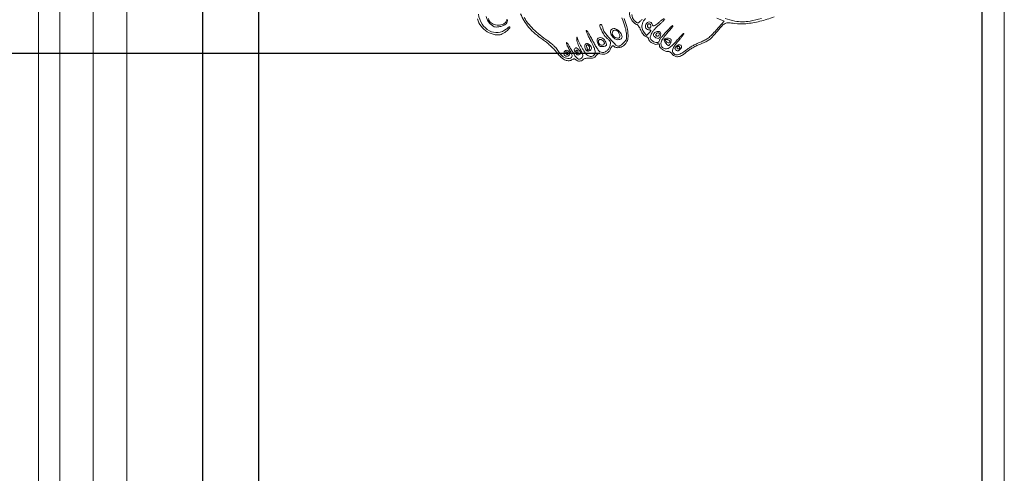
# Model space of a CAD drawing. Units: inches. Extents: x 2656 to 9931, y 1941 to 3068.
# Tile 31 of 46: x 2817 to 2868, y 2929 to 2952. Entities that reach past the tile are written whole.
import ezdxf

# ---------------------------------------------------------------- set-up
doc = ezdxf.new("R2010")
doc.units = ezdxf.units.IN
for name, color, linetype, lineweight in [('A-ANNO-DIMS', 2, 'Continuous', 18), ('A-ELEV-FNSH', 8, 'Continuous', 13), ('A-ELEV-ORN', 8, 'Continuous', 13)]:
    doc.layers.add(name, color=color, linetype=linetype, lineweight=lineweight)
doc.styles.get("Standard").update_dxf_attribs({"font": 'arial.ttf'})
doc.dimstyles.new('ISO-25', dxfattribs={"dimtxt": 6, "dimasz": 2.5, "dimexe": 1.25, "dimexo": 0.625, "dimtad": 1, "dimdec": 0, "dimlunit": 3, "dimtxsty": 'Standard', "dimcen": 2.5, "dimadec": 0, "dimazin": 0, "dimtfac": 1, "dimtdec": 0, "dimtmove": 0, "dimatfit": 3, "dimfxl": 1, "dimarcsym": 0})

# ---------------------------------------------------------------- blocks, each defined once
blk = doc.blocks.new('*D151')
at = {"layer": 'A-ANNO-DIMS', "color": 0, "lineweight": -2, "transparency": 16777216}
for p, q in [((2829.546, 2956.424), (2829.546, 2703.709)), ((2867.059, 2955.98), (2867.059, 2703.709)), ((2832.046, 2704.959), (2864.559, 2704.959))]:
    blk.add_line(p, q, dxfattribs=at)
at = {"layer": 'A-ANNO-DIMS', "color": 0, "transparency": 16777216}
for points in [[(2832.046, 2705.376), (2832.046, 2704.543), (2829.546, 2704.959)], [(2864.559, 2705.376), (2864.559, 2704.543), (2867.059, 2704.959)]]:
    blk.add_solid(points, dxfattribs=at)
at = {"layer": 'Defpoints', "color": 0, "transparency": 16777216}
for p in [(2829.546, 2957.049), (2867.059, 2956.605), (2867.059, 2704.959)]:
    blk.add_point(p, dxfattribs=at)
at = {"layer": 'A-ANNO-DIMS', "color": 0, "transparency": 16777216, "insert": (2848.302, 2708.689), "char_height": 6, "attachment_point": 5}
blk.add_mtext('3\'-1 1/2"', dxfattribs=at)
blk = doc.blocks.new('*D152')
at = {"layer": 'A-ANNO-DIMS', "color": 0, "lineweight": -2, "transparency": 16777216}
for p, q in [((2847.28, 2990.828), (2707.323, 2990.828)), ((2708.573, 2988.328), (2708.573, 2952.971)), ((2847.248, 2950.471), (2707.323, 2950.471))]:
    blk.add_line(p, q, dxfattribs=at)
at = {"layer": 'A-ANNO-DIMS', "color": 0, "transparency": 16777216}
for points in [[(2708.156, 2988.328), (2708.989, 2988.328), (2708.573, 2990.828)], [(2708.156, 2952.971), (2708.989, 2952.971), (2708.573, 2950.471)]]:
    blk.add_solid(points, dxfattribs=at)
at = {"layer": 'Defpoints', "color": 0, "transparency": 16777216}
for p in [(2847.905, 2990.828), (2708.573, 2950.471), (2847.873, 2950.471)]:
    blk.add_point(p, dxfattribs=at)
at = {"layer": 'A-ANNO-DIMS', "color": 0, "transparency": 16777216, "insert": (2704.843, 2970.649), "char_height": 6, "attachment_point": 5, "rotation": 90}
blk.add_mtext('3\'-4 1/2"', dxfattribs=at)
blk = doc.blocks.new('*D153')
at = {"layer": 'A-ANNO-DIMS', "color": 0, "lineweight": -2, "transparency": 16777216}
for p, q in [((2826.64, 2993.722), (2826.64, 2703.709)), ((2829.546, 2956.424), (2829.546, 2703.709)), ((2824.14, 2704.959), (2821.64, 2704.959)), ((2826.64, 2704.959), (2829.546, 2704.959)), ((2832.046, 2704.959), (2851.745, 2704.959))]:
    blk.add_line(p, q, dxfattribs=at)
at = {"layer": 'A-ANNO-DIMS', "color": 0, "transparency": 16777216}
for points in [[(2824.14, 2705.376), (2824.14, 2704.543), (2826.64, 2704.959)], [(2832.046, 2705.376), (2832.046, 2704.543), (2829.546, 2704.959)]]:
    blk.add_solid(points, dxfattribs=at)
at = {"layer": 'Defpoints', "color": 0, "transparency": 16777216}
for p in [(2826.64, 2994.347), (2829.546, 2957.049), (2829.546, 2704.959)]:
    blk.add_point(p, dxfattribs=at)
at = {"layer": 'A-ANNO-DIMS', "color": 0, "transparency": 16777216, "insert": (2843.145, 2708.65), "char_height": 6, "attachment_point": 5}
blk.add_mtext('0\'-3"', dxfattribs=at)

msp = doc.modelspace()

# ---------------------------------------------------------------- linework, layer by layer
at = {"layer": 'A-ELEV-FNSH'}
for p, q in [((2818.129, 2887.893), (2818.129, 2998.286)), ((2819.227, 2887.893), (2819.227, 2998.286)), ((2820.954, 2887.893), (2820.954, 2998.286)), ((2822.705, 2887.893), (2822.705, 2998.286))]:
    msp.add_line(p, q, dxfattribs=at)
msp.add_lwpolyline([(2826.64, 2994.347), (2868.226, 2994.347), (2868.226, 2892.035), (2826.64, 2892.035)], close=True, dxfattribs=at)
at = {"layer": 'A-ELEV-ORN'}
for points in [[(2848.801, 2952.672, 0.216659), (2848.924, 2952.173, 0.024142), (2848.989, 2952.098, 0.029169), (2849.056, 2952.036, 0.030018), (2849.118, 2951.991, 0.14114), (2849.16, 2951.978, -0.206861), (2849.199, 2951.961, -0.032643), (2849.253, 2951.894, -0.031638), (2849.311, 2951.801, -0.022863), (2849.363, 2951.691, 0.032088), (2849.421, 2951.575, 0.039321), (2849.49, 2951.475, 0.044219), (2849.561, 2951.401, 0.114242), (2849.627, 2951.367, -0.05877), (2849.681, 2951.346, -0.064566), (2849.728, 2951.313, -0.073322), (2849.759, 2951.273, -0.133163), (2849.77, 2951.234, 0.196142), (2849.812, 2951.132, 0.063805), (2849.942, 2951.029, 0.063115), (2850.097, 2950.961, 0.16535), (2850.217, 2950.965, -0.060457), (2850.268, 2950.978, -0.16436), (2850.304, 2950.971, -0.184298), (2850.325, 2950.944, -0.078925), (2850.333, 2950.898, 0.185704), (2850.373, 2950.794, 0.054155), (2850.503, 2950.678, 0.054153), (2850.655, 2950.593, 0.183335), (2850.767, 2950.588, -0.170308), (2850.81, 2950.587, -0.049123), (2850.872, 2950.558, -0.043275), (2850.94, 2950.508, -0.034537), (2851.003, 2950.443, 0.112897), (2851.154, 2950.332, 0.151039), (2851.321, 2950.314, 0.097306), (2851.525, 2950.396, 0.029789), (2851.794, 2950.595, -0.032237), (2851.932, 2950.696, -0.016051), (2852.119, 2950.806, -0.015862), (2852.32, 2950.909, -0.022458), (2852.506, 2950.986, 0.023761), (2852.744, 2951.086, 0.048062), (2852.919, 2951.191, 0.044595), (2853.078, 2951.332, 0.017836), (2853.27, 2951.551, -0.01156), (2853.571, 2951.903, -0.094216), (2853.738, 2952.03, -0.127885), (2853.919, 2952.069, -0.028057), (2854.239, 2952.037, 0.065509), (2854.825, 2952.022, 0.033923), (2855.548, 2952.148, 0.033055), (2856.284, 2952.381, 0.043026)], [(2840.893, 2952.277, 0.097952), (2841.082, 2951.892, 0.097989), (2841.403, 2951.609, 0.086415), (2841.822, 2951.453, 0.039063), (2841.956, 2951.439, 0.065886), (2842.068, 2951.451, 0.061015), (2842.178, 2951.492, 0.028884), (2842.309, 2951.57, 0.020818), (2842.404, 2951.64, 0.022925), (2842.489, 2951.715, 0.023115), (2842.555, 2951.786, 0.097823), (2842.584, 2951.836, 0.416465), (2842.574, 2951.856, 0.186344), (2842.542, 2951.854, 0.050913), (2842.477, 2951.816, 0.01734), (2842.39, 2951.748, -0.149603), (2841.966, 2951.568, -0.150262), (2841.514, 2951.656, -0.129848), (2841.142, 2952.002, -0.100707), (2840.945, 2952.522, -0.033876)], [(2841.353, 2952.403, 0.154333), (2841.544, 2952.035, 0.024688), (2841.669, 2951.922, 0.082141), (2841.765, 2951.867, 0.092986), (2841.866, 2951.849, 0.037226), (2842.007, 2951.862, 0.038366), (2842.202, 2951.909, 0.07779), (2842.341, 2951.979, 0.107669), (2842.424, 2952.071, 0.139876), (2842.451, 2952.181, 0.032838), (2842.446, 2952.228, 0.51286), (2842.433, 2952.234, 0.163716), (2842.416, 2952.216, 0.010729), (2842.386, 2952.146, -0.203512), (2842.242, 2952.003, -0.096781), (2841.981, 2951.952, -0.091076), (2841.705, 2952.003, -0.155421), (2841.524, 2952.148, -0.129288), (2841.477, 2952.285, -0.032632)], [(2843.136, 2952.533, 0.048744), (2843.312, 2952.178, 0.037984), (2843.567, 2951.831, 0.035321), (2843.893, 2951.502, 0.029786), (2844.28, 2951.201, -0.019345), (2844.472, 2951.059, -0.014584), (2844.672, 2950.888, -0.014803), (2844.851, 2950.716, -0.032702), (2844.974, 2950.572, 0.035674), (2845.196, 2950.317, 0.072427), (2845.41, 2950.158, 0.10378), (2845.604, 2950.101, 0.161146), (2845.773, 2950.142, -0.035481), (2845.845, 2950.18, -0.087902), (2845.902, 2950.194, -0.117123), (2845.951, 2950.186, -0.096474), (2845.994, 2950.156, 0.107887), (2846.08, 2950.101, 0.095562), (2846.186, 2950.083, 0.093343), (2846.292, 2950.106, 0.097186), (2846.381, 2950.166, -0.108118), (2846.431, 2950.198, -0.038631), (2846.512, 2950.221, -0.036146), (2846.608, 2950.233, -0.035408), (2846.705, 2950.232, 0.035182), (2846.823, 2950.23, 0.075501), (2846.912, 2950.248, 0.087997), (2846.983, 2950.29, 0.063219), (2847.045, 2950.358, -0.05042), (2847.096, 2950.417, -0.079909), (2847.151, 2950.455, -0.095326), (2847.208, 2950.47, -0.106795), (2847.263, 2950.461, 0.103678), (2847.42, 2950.436, 0.099264), (2847.576, 2950.475, 0.095648), (2847.71, 2950.573, 0.088752), (2847.802, 2950.716, -0.023551), (2847.847, 2950.812, -0.092945), (2847.888, 2950.863, -0.202519), (2847.926, 2950.876, -0.176634), (2847.965, 2950.858, 0.148207), (2848.095, 2950.789, 0.097714), (2848.265, 2950.788, 0.087841), (2848.438, 2950.855, 0.090106), (2848.576, 2950.977, 0.044786), (2848.653, 2951.094, 0.069827), (2848.694, 2951.207, 0.054055), (2848.708, 2951.347, 0.017152), (2848.7, 2951.557, 0.049543), (2848.643, 2951.884, 0.023015), (2848.508, 2952.294, 0.022134)], [(2848.393, 2952.319, -0.01692), (2848.543, 2951.895, -0.043427), (2848.613, 2951.578, -0.015509), (2848.635, 2951.365, -0.077549), (2848.625, 2951.245, -0.100968), (2848.58, 2951.149, -0.035807), (2848.48, 2951.035, -0.019689), (2848.405, 2950.965, -0.02395), (2848.33, 2950.907, -0.023531), (2848.263, 2950.865, -0.129915), (2848.222, 2950.854, -0.20167), (2848.082, 2950.912, -0.012833), (2847.774, 2951.244, -0.016262), (2847.489, 2951.588, -0.115769), (2847.4, 2951.784, 0.028588), (2847.381, 2951.859, 0.041166), (2847.354, 2951.922, 0.047726), (2847.326, 2951.966, 0.229861), (2847.299, 2951.979, 0.186476), (2847.258, 2951.963, 0.246151), (2847.244, 2951.926, 0.060512), (2847.265, 2951.845, 0.005494), (2847.343, 2951.653, 0.03364), (2847.396, 2951.547, 0.023761), (2847.469, 2951.435, 0.02409), (2847.549, 2951.335, 0.045688), (2847.624, 2951.264, -0.049294), (2847.74, 2951.152, -0.129909), (2847.79, 2951.049, -0.118001), (2847.785, 2950.928, -0.037071), (2847.722, 2950.758, -0.093173), (2847.636, 2950.636, -0.099676), (2847.513, 2950.557, -0.104799), (2847.375, 2950.534, -0.113979), (2847.244, 2950.57, -0.113308), (2847.186, 2950.621, -0.011986), (2847.085, 2950.77, -0.014319), (2846.972, 2950.956, -0.011031), (2846.859, 2951.166, 0.007389), (2846.751, 2951.369, 0.012759), (2846.655, 2951.534, 0.006744), (2846.572, 2951.664, 0.475628), (2846.55, 2951.666, 0.298473), (2846.543, 2951.636, 0.005773), (2846.605, 2951.485, 0.011889), (2846.685, 2951.306, 0.007437), (2846.787, 2951.101, -0.008452), (2846.924, 2950.823, -0.037472), (2846.99, 2950.653, -0.069448), (2847.008, 2950.536, -0.145257), (2846.983, 2950.448, -0.146465), (2846.856, 2950.337, -0.198924), (2846.705, 2950.332, -0.123587), (2846.539, 2950.447, -0.046452), (2846.372, 2950.678, -0.009207), (2846.288, 2950.825, -0.008845), (2846.209, 2950.978, -0.008807), (2846.143, 2951.115, -0.0314), (2846.109, 2951.205, 0.002514), (2846.074, 2951.317, 0.226761), (2846.062, 2951.33, 0.508235), (2846.053, 2951.324, 0.004483), (2846.048, 2951.229, 0.07523), (2846.057, 2951.147, 0.017337), (2846.098, 2951.014, 0.017529), (2846.156, 2950.862, 0.016323), (2846.226, 2950.711, -0.008903), (2846.33, 2950.495, -0.068964), (2846.362, 2950.387, -0.146939), (2846.351, 2950.312, -0.089299), (2846.299, 2950.237, -0.17255), (2846.191, 2950.185, -0.201973), (2846.083, 2950.218, -0.077507), (2845.955, 2950.364, -0.013086), (2845.764, 2950.684, 0.008257), (2845.622, 2950.925, 0.047089), (2845.533, 2951.044, 0.715316), (2845.51, 2951.034, 0.071182), (2845.53, 2950.942, 0.021409), (2845.557, 2950.879, 0.006729), (2845.602, 2950.788, 0.006709), (2845.655, 2950.688, 0.007384), (2845.71, 2950.592, -0.041313), (2845.792, 2950.421, -0.176517), (2845.794, 2950.309, -0.238643), (2845.726, 2950.243, -0.075156), (2845.581, 2950.221, -0.103457), (2845.441, 2950.25, -0.071525), (2845.303, 2950.335, -0.055375), (2845.166, 2950.479, -0.028769), (2845.026, 2950.686, 0.053224), (2844.955, 2950.781, 0.018463), (2844.834, 2950.902, 0.0181), (2844.69, 2951.026, 0.020079), (2844.542, 2951.135, -0.021598), (2844.142, 2951.432, -0.025464), (2843.792, 2951.747, -0.027925), (2843.511, 2952.059, -0.051755), (2843.327, 2952.345, -0.041492)], [(2849.443, 2952.253, -0.031818), (2849.345, 2952.153, -0.02297), (2849.253, 2952.076, -0.18391), (2849.201, 2952.061, -0.160327), (2849.148, 2952.084, -0.016424), (2849.048, 2952.178, -0.185893), (2848.905, 2952.5, -0.094612)], [(2850.574, 2952.297, 0.028686), (2850.476, 2952.229, 0.011691), (2850.351, 2952.127, -0.006102), (2850.146, 2951.956, -0.080138), (2850.061, 2951.907, -0.286715), (2850.008, 2951.918, -0.11616), (2849.966, 2951.981, 0.117291), (2849.902, 2952.078, 0.182702), (2849.811, 2952.115, 0.173341), (2849.714, 2952.083, 0.105255), (2849.635, 2951.99, 0.123366), (2849.609, 2951.886, 0.148353), (2849.638, 2951.789, 0.140375), (2849.718, 2951.722, 0.106459), (2849.83, 2951.698, -0.097174), (2849.872, 2951.69, -0.360986), (2849.884, 2951.667, -0.11978), (2849.865, 2951.627, -0.014081), (2849.8, 2951.552), (2849.668, 2951.405), (2849.543, 2951.559, -0.11694), (2849.432, 2951.789, -0.142406), (2849.449, 2952.027, -0.093777), (2849.607, 2952.292, -0.031312)], [(2853.322, 2952.304), (2853.698, 2952.151), (2853.279, 2951.683, -0.014019), (2853.048, 2951.439, -0.035056), (2852.863, 2951.278, -0.042181), (2852.679, 2951.163, -0.030354), (2852.458, 2951.065, 0.020169), (2852.285, 2950.992, 0.014439), (2852.097, 2950.899, 0.014617), (2851.924, 2950.799, 0.030123), (2851.796, 2950.708, -0.023096), (2851.542, 2950.525, -0.065579), (2851.346, 2950.43, -0.108644), (2851.194, 2950.415, -0.169259), (2851.076, 2950.472, -0.14578), (2851.018, 2950.581, -0.143269), (2851.027, 2950.705, -0.069423), (2851.119, 2950.873, -0.01412), (2851.33, 2951.14, 0.007738), (2851.433, 2951.267, 0.011134), (2851.52, 2951.382, 0.007109), (2851.588, 2951.481, 0.149256), (2851.599, 2951.515, 0.659704), (2851.585, 2951.521, 0.007404), (2851.49, 2951.427, 0.010983), (2851.371, 2951.301, 0.005888), (2851.229, 2951.141, -0.022729), (2850.977, 2950.874, -0.083791), (2850.786, 2950.743, -0.155343), (2850.629, 2950.723, -0.15181), (2850.487, 2950.797, -0.144109), (2850.418, 2950.924, -0.132791), (2850.426, 2951.073, -0.077589), (2850.521, 2951.26, -0.023454), (2850.719, 2951.509, 0.002598), (2851.017, 2951.853, 0.277519), (2851.026, 2951.911, 0.545774), (2850.99, 2951.918, 0.002794), (2850.684, 2951.599, 0.009193), (2850.55, 2951.451, 0.013114), (2850.436, 2951.315, 0.009044), (2850.347, 2951.198, 0.159361), (2850.333, 2951.153, -0.217862), (2850.298, 2951.077, -0.162357), (2850.211, 2951.041, -0.109971), (2850.09, 2951.06, -0.078028), (2849.972, 2951.128, -0.033256), (2849.885, 2951.209, -0.145423), (2849.854, 2951.271, -0.122821), (2849.858, 2951.345, -0.020849), (2849.908, 2951.48, -0.053925), (2849.964, 2951.583, -0.021987), (2850.062, 2951.711, -0.021448), (2850.179, 2951.84, -0.02561), (2850.301, 2951.951, 0.013398), (2850.419, 2952.053, 0.015652), (2850.525, 2952.156, 0.014705), (2850.609, 2952.248, 0.085937)], [(2855.626, 2952.288, -0.01477), (2855.041, 2952.158, -0.047431), (2854.644, 2952.12, -0.052476), (2854.249, 2952.161, -0.023008), (2853.739, 2952.294, -0.023068)]]:
    msp.add_lwpolyline(points, format="xyb", dxfattribs=at)
for points in [[(2847.847, 2951.721, 0.251131), (2847.798, 2951.559, 0.124898), (2847.894, 2951.359, 0.113091), (2848.082, 2951.216, 0.200091), (2848.274, 2951.21, 0.048277), (2848.344, 2951.245, 0.117693), (2848.384, 2951.286, 0.140447), (2848.397, 2951.335, 0.081949), (2848.387, 2951.396, 0.077801), (2848.283, 2951.587, 0.09434), (2848.132, 2951.723, 0.124914), (2847.974, 2951.77, 0.210773)], [(2848.22, 2951.562, -0.03358), (2848.28, 2951.43, -0.141285), (2848.286, 2951.344, -0.241436), (2848.246, 2951.294, -0.105107), (2848.161, 2951.276, -0.117324), (2848.044, 2951.304, -0.10171), (2847.945, 2951.382, -0.109775), (2847.89, 2951.487, -0.158111), (2847.896, 2951.591, -0.149626), (2847.957, 2951.669, -0.177198), (2848.047, 2951.693, -0.148121), (2848.144, 2951.654, -0.100327)], [(2849.875, 2951.838, -0.074012), (2849.849, 2951.807, -0.156529), (2849.82, 2951.794, -0.15302), (2849.788, 2951.801, -0.06978), (2849.754, 2951.826, -0.088981), (2849.731, 2951.859, -0.076381), (2849.719, 2951.9, -0.077007), (2849.721, 2951.942, -0.093176), (2849.735, 2951.979, -0.074012), (2849.761, 2952.011, -0.156529), (2849.791, 2952.023, -0.15302), (2849.822, 2952.017, -0.06978), (2849.856, 2951.991, -0.088981), (2849.879, 2951.958, -0.076381), (2849.891, 2951.917, -0.077007), (2849.89, 2951.875, -0.093176)], [(2847.166, 2951.275, 0.095208), (2847.122, 2951.235, 0.133582), (2847.103, 2951.185, 0.088345), (2847.108, 2951.117, 0.025322), (2847.139, 2951.016, 0.039226), (2847.182, 2950.92, 0.106844), (2847.231, 2950.865, 0.12504), (2847.293, 2950.839, 0.064245), (2847.378, 2950.838, 0.021524), (2847.516, 2950.859, 0.175493), (2847.569, 2950.892, 0.215239), (2847.583, 2950.947, 0.033952), (2847.556, 2951.06, 0.092865), (2847.491, 2951.18, 0.097317), (2847.388, 2951.267, 0.110796), (2847.271, 2951.301, 0.15554)], [(2847.441, 2951.109, -0.052573), (2847.475, 2951.059, -0.14188), (2847.483, 2951.017, -0.144742), (2847.468, 2950.978, -0.055548), (2847.427, 2950.935, -0.17181), (2847.345, 2950.905, -0.155184), (2847.258, 2950.931, -0.13098), (2847.191, 2951.009, -0.112001), (2847.168, 2951.114, -0.218344), (2847.197, 2951.177, -0.184093), (2847.266, 2951.202, -0.123773), (2847.359, 2951.177, -0.092306)], [(2850.06, 2951.533, 0.078467), (2850.029, 2951.481, 0.152913), (2850.026, 2951.433, 0.116494), (2850.05, 2951.384, 0.035989), (2850.109, 2951.323, 0.119877), (2850.213, 2951.266, 0.20352), (2850.31, 2951.28, 0.172143), (2850.379, 2951.364, 0.086245), (2850.403, 2951.501, 0.208669), (2850.366, 2951.585, 0.165357), (2850.275, 2951.626, 0.127666), (2850.158, 2951.606, 0.116165)], [(2850.333, 2951.498, -0.108877), (2850.319, 2951.438, -0.127543), (2850.282, 2951.393, -0.144342), (2850.232, 2951.375, -0.153624), (2850.181, 2951.388, -0.216101), (2850.152, 2951.431, -0.159804), (2850.161, 2951.489, -0.132181), (2850.205, 2951.539, -0.145303), (2850.266, 2951.557, -0.087308), (2850.292, 2951.553, -0.094392), (2850.313, 2951.54, -0.100145), (2850.328, 2951.521, -0.112153)], [(2850.58, 2951.208, 0.193695), (2850.574, 2951.172, 0.058266), (2850.592, 2951.119, 0.048819), (2850.629, 2951.058, 0.036452), (2850.68, 2950.999, 0.010243), (2850.775, 2950.907, 0.186958), (2850.813, 2950.892, 0.256873), (2850.845, 2950.91, 0.019698), (2850.897, 2950.997, 0.040391), (2850.923, 2951.056, 0.043863), (2850.938, 2951.117, 0.048392), (2850.941, 2951.171, 0.129399), (2850.93, 2951.207, 0.180632), (2850.865, 2951.257, 0.074944), (2850.755, 2951.274, 0.075027), (2850.645, 2951.257, 0.182191)], [(2850.857, 2951.14, -0.189332), (2850.869, 2951.076, -0.296611), (2850.831, 2951.037, -0.169397), (2850.755, 2951.045, -0.107759), (2850.684, 2951.101, -0.020503), (2850.641, 2951.157, -0.209835), (2850.635, 2951.185, -0.309419), (2850.652, 2951.201, -0.038489), (2850.707, 2951.205, -0.053722), (2850.752, 2951.201, -0.048999), (2850.796, 2951.186, -0.052232), (2850.834, 2951.165, -0.09982)], [(2845.386, 2950.542, 0.166245), (2845.382, 2950.451, 0.151719), (2845.435, 2950.372, 0.149289), (2845.524, 2950.337, 0.16055), (2845.615, 2950.358, 0.190949), (2845.668, 2950.429, 0.143859), (2845.666, 2950.528, 0.139493), (2845.61, 2950.611, 0.178716), (2845.524, 2950.643, 0.090292), (2845.483, 2950.635, 0.066647), (2845.442, 2950.613, 0.065393), (2845.408, 2950.581, 0.079367)], [(2845.938, 2950.715, 0.198865), (2845.922, 2950.619, 0.09268), (2845.974, 2950.502, 0.097846), (2846.062, 2950.416, 0.240946), (2846.149, 2950.407, 0.087263), (2846.223, 2950.451, 0.223388), (2846.248, 2950.507, 0.153424), (2846.224, 2950.578, 0.038406), (2846.143, 2950.673, 0.013143), (2846.056, 2950.755, 0.133914), (2846.013, 2950.777, 0.254303), (2845.978, 2950.766, 0.055423)], [(2846.113, 2950.572, -0.042167), (2846.11, 2950.545, -0.061769), (2846.103, 2950.523, -0.081139), (2846.093, 2950.507, -0.210953), (2846.082, 2950.502, -0.151918), (2846.067, 2950.507, -0.038439), (2846.047, 2950.523, -0.035638), (2846.026, 2950.545, -0.029505), (2846.007, 2950.572, -0.082592), (2845.996, 2950.599, -0.161196), (2845.998, 2950.622, -0.182303), (2846.013, 2950.637, -0.108972), (2846.038, 2950.643, -0.093332), (2846.066, 2950.637, -0.09642), (2846.091, 2950.622, -0.099167), (2846.107, 2950.599, -0.105053)], [(2846.465, 2950.871, 0.065921), (2846.483, 2950.744, 0.11591), (2846.534, 2950.651, 0.153891), (2846.61, 2950.607, 0.149294), (2846.698, 2950.613, 0.107755), (2846.777, 2950.664, 0.167613), (2846.811, 2950.737, 0.147269), (2846.796, 2950.822, 0.077976), (2846.731, 2950.91, 0.080544), (2846.64, 2950.976, 0.15324), (2846.551, 2950.99, 0.211421), (2846.489, 2950.951, 0.151601)], [(2846.7, 2950.821, -0.066719), (2846.71, 2950.778, -0.072258), (2846.708, 2950.736, -0.081026), (2846.695, 2950.7, -0.126981), (2846.672, 2950.676, -0.034732), (2846.646, 2950.662, -0.074198), (2846.625, 2950.657, -0.143207), (2846.611, 2950.659, -0.287633), (2846.605, 2950.668, 0.061959), (2846.602, 2950.687, 0.00979), (2846.592, 2950.724, 0.010735), (2846.579, 2950.768, 0.009199), (2846.562, 2950.813, -0.054634), (2846.551, 2950.855, -0.098218), (2846.553, 2950.891, -0.14605), (2846.567, 2950.915, -0.188995), (2846.59, 2950.924, -0.125056), (2846.62, 2950.917, -0.064167), (2846.651, 2950.894, -0.057615), (2846.679, 2950.86, -0.055112)], [(2851.184, 2950.828, 0.053545), (2851.151, 2950.777, 0.143201), (2851.143, 2950.735, 0.143819), (2851.158, 2950.696, 0.054184), (2851.2, 2950.652, 0.077176), (2851.253, 2950.621, 0.154286), (2851.3, 2950.617, 0.117177), (2851.35, 2950.642, 0.035256), (2851.412, 2950.701, 0.060425), (2851.475, 2950.791, 0.19481), (2851.483, 2950.862, 0.240731), (2851.44, 2950.908, 0.087827), (2851.349, 2950.924, 0.088999), (2851.311, 2950.917, 0.043202), (2851.266, 2950.896, 0.041019), (2851.221, 2950.865, 0.046615)], [(2851.388, 2950.783, -0.099038), (2851.382, 2950.757, -0.097945), (2851.367, 2950.734, -0.097945), (2851.344, 2950.718, -0.099038), (2851.317, 2950.713, -0.099038), (2851.29, 2950.718, -0.097945), (2851.268, 2950.734, -0.097945), (2851.252, 2950.757, -0.099038), (2851.247, 2950.783, -0.099038), (2851.252, 2950.81, -0.097945), (2851.268, 2950.833, -0.097945), (2851.29, 2950.848, -0.099038), (2851.317, 2950.854, -0.099038), (2851.344, 2950.848, -0.097945), (2851.367, 2950.833, -0.097945), (2851.382, 2950.81, -0.099038)], [(2845.585, 2950.502, -0.082592), (2845.596, 2950.475, -0.161196), (2845.594, 2950.452, -0.182303), (2845.579, 2950.437, -0.108972), (2845.554, 2950.432, -0.093332), (2845.526, 2950.437, -0.09642), (2845.501, 2950.452, -0.099167), (2845.485, 2950.475, -0.105053), (2845.48, 2950.502, -0.042167), (2845.482, 2950.529, -0.061769), (2845.489, 2950.552, -0.081139), (2845.499, 2950.567, -0.210953), (2845.511, 2950.572, -0.151918), (2845.525, 2950.568, -0.038439), (2845.545, 2950.552, -0.035638), (2845.566, 2950.529, -0.029505)]]:
    msp.add_lwpolyline(points, format="xyb", close=True, dxfattribs=at)

# ---------------------------------------------------------------- dimensions: what is measured, and where the dimension line sits
at = {"layer": 'A-ANNO-DIMS'}
for base, p1, p2, picture, middle in [((2829.546, 2704.959), (2826.64, 2994.347), (2829.546, 2957.049), '*D153', (2843.145, 2708.65)), ((2867.059, 2704.959), (2829.546, 2957.049), (2867.059, 2956.605), '*D151', (2848.302, 2708.689))]:
    dim = msp.add_linear_dim(base=base, p1=p1, p2=p2, dimstyle='ISO-25', override={"dimdec": 1, "dimlfac": 1, "dimrnd": 0, "dimzin": 1, "dimdsep": 46, "dimlunit": 4, "dimfrac": 2}, dxfattribs=at)
    dim.commit()
    dim.dimension.update_dxf_attribs({"geometry": picture, "text_midpoint": middle})
dim = msp.add_linear_dim(base=(2708.573, 2950.471), p1=(2847.905, 2990.828), p2=(2847.873, 2950.471), angle=90, dimstyle='ISO-25', override={"dimdec": 1, "dimlfac": 1, "dimrnd": 0, "dimzin": 1, "dimdsep": 46, "dimlunit": 4, "dimfrac": 2}, dxfattribs=at)
dim.commit()
dim.dimension.update_dxf_attribs({"geometry": '*D152', "text_midpoint": (2704.843, 2970.649)})

doc.saveas('drawing.dxf')
